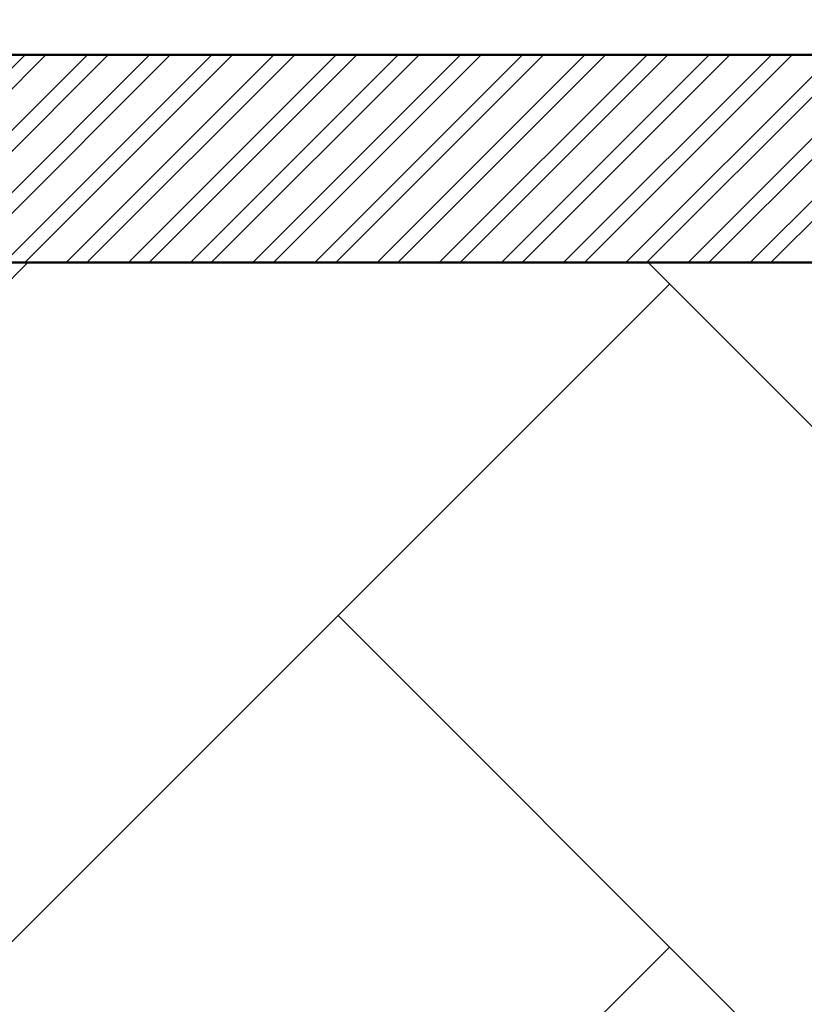
# Model space of a CAD drawing. Units: inches. Extents: x 3590 to 5167, y 65 to 1917.
# Tile 71 of 100: x 5001 to 5035, y 1765 to 1808. Entities that reach past the tile are written whole.
import ezdxf

# ---------------------------------------------------------------- set-up
doc = ezdxf.new("R2010")
doc.units = ezdxf.units.IN
for name, color, linetype, lineweight in [('A-ANNO-DIMS', 2, 'Continuous', 18), ('A-FLOR-PATT', 8, 'Continuous', 13), ('A-WALL', 7, 'Continuous', 50), ('A-WALL-PATT', 251, 'Continuous', 13)]:
    doc.layers.add(name, color=color, linetype=linetype, lineweight=lineweight)
doc.styles.get("Standard").update_dxf_attribs({"font": 'arial.ttf'})
doc.dimstyles.new('ISO-25', dxfattribs={"dimtxt": 9, "dimasz": 2.5, "dimexe": 1.25, "dimexo": 0.625, "dimtad": 1, "dimdec": 1, "dimlunit": 3, "dimtxsty": 'Standard', "dimcen": 2.5, "dimadec": 0, "dimazin": 0, "dimtfac": 1, "dimtdec": 1, "dimtmove": 0, "dimatfit": 3, "dimfxl": 1, "dimarcsym": 0})

# ---------------------------------------------------------------- blocks, each defined once
blk = doc.blocks.new('*D101')
at = {"layer": 'A-ANNO-DIMS', "color": 0, "lineweight": -2, "transparency": 16777216}
for p, q in [((4420.274, 1806.624), (4420.274, 1818.615)), ((5080.274, 1806.624), (5080.274, 1818.615)), ((4422.774, 1817.365), (5077.774, 1817.365))]:
    blk.add_line(p, q, dxfattribs=at)
at = {"layer": 'A-ANNO-DIMS', "color": 0, "transparency": 16777216}
for points in [[(4422.774, 1817.781), (4422.774, 1816.948), (4420.274, 1817.365)], [(5077.774, 1817.781), (5077.774, 1816.948), (5080.274, 1817.365)]]:
    blk.add_solid(points, dxfattribs=at)
at = {"layer": 'Defpoints', "color": 0, "transparency": 16777216}
for p in [(5080.274, 1817.365), (4420.274, 1805.999), (5080.274, 1805.999)]:
    blk.add_point(p, dxfattribs=at)
at = {"layer": 'A-ANNO-DIMS', "color": 0, "transparency": 16777216, "insert": (4750.274, 1822.566), "char_height": 9, "attachment_point": 5}
blk.add_mtext("55'", dxfattribs=at)

msp = doc.modelspace()

# ---------------------------------------------------------------- hatches: boundary and pattern name
at = {"layer": 'A-FLOR-PATT', "transparency": 33554687}
h = msp.add_hatch(dxfattribs=at)
h.set_pattern_fill('AR-HBONE', color=256, scale=0.2)
h.set_pattern_definition([(45, (-588.972, 0), (0, 28.73682), [60.96, -20.32]), (135, (-574.604, 14.368), (3e-15, 28.73682), [60.96, -20.32])])
h.paths.add_polyline_path([(5071.274, 1796.999), (4933.274, 1796.999), (4933.274, 1753.999), (4962.774, 1753.999, -0.414214), (4928.774, 1719.999), (4933.274, 1718.999), (4933.274, 1334.999), (5071.274, 1334.999)])
h.paths.add_polyline_path([(4951.78, 1521.077), (4951.715, 1521.04), (4951.563, 1520.895)], flags=16)
h.paths.add_polyline_path([(4952.267, 1521.376), (4952.198, 1521.371), (4952.198, 1521.356)], flags=0)
h.paths.add_polyline_path([(4967.051, 1529.728), (4965.231, 1528.694), (4963.411, 1527.714), (4961.756, 1526.851), (4963.589, 1527.449), (4964.036, 1527.478), (4962.975, 1527.249), (4961.76, 1526.852), (4959.792, 1525.834), (4958.005, 1524.895), (4956.24, 1523.93), (4954.504, 1522.919), (4954.129, 1522.682), (4953.361, 1521.997), (4953.366, 1521.998), (4953.605, 1522.064), (4955.106, 1522.761), (4956.921, 1523.434), (4958.678, 1523.915), (4960.358, 1524.2), (4961.945, 1524.286), (4964.171, 1524.108), (4965.958, 1523.309), (4963.863, 1522.976), (4965.187, 1522.499), (4963.366, 1522.497), (4961.545, 1522.487), (4959.764, 1522.461), (4958.304, 1522.419), (4957.974, 1522.388), (4956.307, 1522.232), (4954.718, 1522.071), (4953.251, 1521.899), (4953.525, 1521.623), (4954.331, 1521.379), (4956.243, 1521.23), (4958.039, 1520.93), (4959.684, 1520.483), (4961.16, 1519.896), (4963.107, 1518.8), (4964.393, 1517.325), (4962.973, 1517.726), (4964.558, 1516.661), (4965.407, 1515.708), (4963.507, 1516.322), (4961.68, 1517.005), (4959.935, 1517.745), (4958.282, 1518.528), (4956.732, 1519.343), (4955.295, 1520.175), (4954.672, 1520.572), (4954.513, 1520.627), (4955.658, 1519.318), (4956.703, 1517.982), (4957.644, 1516.647), (4958.485, 1515.334), (4959.55, 1513.524), (4960.438, 1511.769), (4958.841, 1513.62), (4957.452, 1515.325), (4955.819, 1517.459), (4956.665, 1515.448), (4957.111, 1513.923), (4957.447, 1511.714), (4957.076, 1509.793), (4956.538, 1511.11), (4955.992, 1512.569), (4955.444, 1514.125), (4954.898, 1515.735), (4954.357, 1517.356), (4953.824, 1518.943), (4953.305, 1520.452), (4953.065, 1521.116), (4952.971, 1521.146), (4952.949, 1521.086), (4952.73, 1520.199), (4953.37, 1518.024), (4953.757, 1516.373), (4954.051, 1514.765), (4954.264, 1513.221), (4954.471, 1511.131), (4954.497, 1510.402), (4954.409, 1511.76), (4954.264, 1513.221), (4954.051, 1514.765), (4953.757, 1516.373), (4953.37, 1518.024), (4952.877, 1519.698), (4952.716, 1520.141), (4952.533, 1519.059), (4952.374, 1517.789), (4952.219, 1516.312), (4952.046, 1514.6), (4951.833, 1512.626), (4951.557, 1510.363), (4951.203, 1512.168), (4950.852, 1514.339), (4950.985, 1516.376), (4951.66, 1518.286), (4952.593, 1520.481), (4952.357, 1521.13), (4951.855, 1520.328), (4950.839, 1518.908), (4949.777, 1517.587), (4948.916, 1516.617), (4948.111, 1515.256), (4947.089, 1513.554), (4945.889, 1511.615), (4946.326, 1513.402), (4946.562, 1514.249), (4945.528, 1513.327), (4944.581, 1512.531), (4946.018, 1514.508), (4947.204, 1516.048), (4947.893, 1517.313), (4949.307, 1518.764), (4950.414, 1519.767), (4950.451, 1519.806), (4952.267, 1521.376), (4951.645, 1521.493), (4950.404, 1521.18), (4948.044, 1520.359), (4946.119, 1519.452), (4944.572, 1518.475), (4943.35, 1517.443), (4941.997, 1515.92), (4941.661, 1515.275), (4942.813, 1516.99), (4944.572, 1518.475), (4946.119, 1519.452), (4948.044, 1520.359), (4950.404, 1521.18), (4951.645, 1521.493), (4949.647, 1521.868), (4948.6, 1521.756), (4947.126, 1521.57), (4945.42, 1521.348), (4943.45, 1521.105), (4941.183, 1520.856), (4942.86, 1521.613), (4943.873, 1522.03), (4942.952, 1521.909), (4941.41, 1521.485), (4939.543, 1520.67), (4938.968, 1520.226), (4940.733, 1521.299), (4942.952, 1521.909), (4943.702, 1522.008), (4945.894, 1522.7), (4947.565, 1522.714), (4948.921, 1522.566), (4951.131, 1522.183), (4950.971, 1522.297), (4948.129, 1523.006), (4946.035, 1523.707), (4944.232, 1524.521), (4942.707, 1525.461), (4941.444, 1526.537), (4940.43, 1527.761), (4939.649, 1529.143), (4941.421, 1528.122), (4943.147, 1527.132), (4944.841, 1526.175), (4946.514, 1525.25), (4948.179, 1524.359), (4948.365, 1524.263), (4946.475, 1526.045), (4945.181, 1527.54), (4944.19, 1529.033), (4943.496, 1530.54), (4943.278, 1531.36), (4942.498, 1531.919), (4943.114, 1531.762), (4942.959, 1533.659), (4944.14, 1531.989), (4944.612, 1531.323), (4946.202, 1530.463), (4947.486, 1529.509), (4948.79, 1528.226), (4950.368, 1526.237), (4949.485, 1528.155), (4948.851, 1530.123), (4948.491, 1532.041), (4948.381, 1533.918), (4948.501, 1535.76), (4948.827, 1537.573), (4949.418, 1535.565), (4949.957, 1533.569), (4950.464, 1531.586), (4950.961, 1529.617), (4951.391, 1527.954), (4951.724, 1530.687), (4952.201, 1532.58), (4952.889, 1534.33), (4953.77, 1535.951), (4954.827, 1537.46), (4954.521, 1535.39), (4954.273, 1533.937), (4955.58, 1535.663), (4956.748, 1536.739), (4956.159, 1534.78), (4955.589, 1532.873), (4955.043, 1531.006), (4954.525, 1529.166), (4954.038, 1527.341), (4953.638, 1525.733), (4953.611, 1525.586), (4953.398, 1524.166), (4953.382, 1524.009), (4954.07, 1525.476), (4954.912, 1527.022), (4956.136, 1528.894), (4957.847, 1530.577), (4959.376, 1531.54), (4958.256, 1530.104), (4957.143, 1528.663), (4956.066, 1527.243), (4955.056, 1525.871), (4954.141, 1524.571), (4953.352, 1523.372), (4953.311, 1523.303), (4953.273, 1522.925), (4953.261, 1522.382), (4954.103, 1523.373), (4954.63, 1524.284), (4955.961, 1526.358), (4957.23, 1528.13), (4958.421, 1529.609), (4960.037, 1531.368), (4961.374, 1532.375), (4962.101, 1532.77), (4961.07, 1531.061), (4959.987, 1529.438), (4958.869, 1527.908), (4958.15, 1527.007), (4959.803, 1528.003), (4961.589, 1528.793), (4963.391, 1529.328), (4965.211, 1529.632)], flags=16)
h.paths.add_polyline_path([(4962.944, 1523.182), (4961.107, 1523.422), (4960.392, 1523.362), (4962.35, 1523.331)], flags=0)
h.paths.add_polyline_path([(5049.541, 1584.551), (5049.476, 1584.515), (5049.325, 1584.37)], flags=16)
h.paths.add_polyline_path([(5050.028, 1584.851), (5049.959, 1584.845), (5049.959, 1584.83)], flags=0)
h.paths.add_polyline_path([(5042.333, 1581.949), (5043.88, 1582.926), (5045.806, 1583.833), (5048.165, 1584.654), (5049.406, 1584.967), (5047.408, 1585.342), (5046.361, 1585.231), (5044.888, 1585.044), (5043.181, 1584.822), (5041.211, 1584.579), (5038.944, 1584.33), (5040.622, 1585.087), (5041.634, 1585.504), (5040.713, 1585.383), (5039.171, 1584.959), (5037.304, 1584.144), (5036.729, 1583.7), (5038.494, 1584.773), (5040.713, 1585.383), (5041.463, 1585.482), (5043.655, 1586.174), (5045.326, 1586.188), (5046.682, 1586.04), (5048.893, 1585.657), (5048.732, 1585.771), (5045.891, 1586.48), (5043.796, 1587.181), (5041.994, 1587.996), (5040.468, 1588.935), (5039.205, 1590.011), (5038.191, 1591.235), (5037.41, 1592.617), (5039.182, 1591.596), (5040.909, 1590.607), (5042.602, 1589.649), (5044.275, 1588.724), (5045.94, 1587.833), (5046.126, 1587.738), (5044.237, 1589.519), (5042.942, 1591.015), (5041.952, 1592.508), (5041.257, 1594.014), (5041.039, 1594.834), (5040.26, 1595.393), (5040.875, 1595.237), (5040.721, 1597.133), (5041.901, 1595.463), (5042.373, 1594.798), (5043.963, 1593.938), (5045.247, 1592.983), (5046.552, 1591.701), (5048.129, 1589.712), (5047.247, 1591.63), (5046.613, 1593.597), (5046.252, 1595.515), (5046.142, 1597.392), (5046.262, 1599.234), (5046.588, 1601.047), (5047.179, 1599.039), (5047.718, 1597.043), (5048.225, 1595.06), (5048.722, 1593.091), (5049.152, 1591.429), (5049.485, 1594.161), (5049.962, 1596.054), (5050.65, 1597.804), (5051.532, 1599.425), (5052.589, 1600.934), (5052.283, 1598.864), (5052.034, 1597.411), (5053.341, 1599.137), (5054.509, 1600.213), (5053.92, 1598.254), (5053.35, 1596.348), (5052.805, 1594.48), (5052.286, 1592.64), (5051.799, 1590.815), (5051.4, 1589.207), (5051.373, 1589.06), (5051.159, 1587.64), (5051.143, 1587.483), (5051.831, 1588.95), (5052.673, 1590.496), (5053.898, 1592.368), (5055.608, 1594.051), (5057.137, 1595.014), (5056.017, 1593.578), (5054.904, 1592.137), (5053.828, 1590.717), (5052.817, 1589.345), (5051.902, 1588.046), (5051.113, 1586.846), (5051.072, 1586.777), (5051.034, 1586.399), (5051.022, 1585.856), (5051.864, 1586.847), (5052.391, 1587.758), (5053.723, 1589.832), (5054.991, 1591.604), (5056.182, 1593.083), (5057.798, 1594.842), (5059.135, 1595.849), (5059.863, 1596.244), (5058.831, 1594.535), (5057.749, 1592.912), (5056.63, 1591.382), (5055.912, 1590.482), (5057.564, 1591.477), (5059.35, 1592.267), (5061.152, 1592.802), (5062.972, 1593.106), (5064.812, 1593.203), (5062.992, 1592.169), (5061.172, 1591.188), (5059.518, 1590.325), (5061.35, 1590.924), (5061.797, 1590.952), (5060.737, 1590.723), (5059.521, 1590.326), (5057.553, 1589.308), (5055.766, 1588.369), (5054.002, 1587.404), (5052.265, 1586.393), (5051.891, 1586.156), (5051.122, 1585.471), (5051.127, 1585.472), (5051.366, 1585.538), (5052.867, 1586.235), (5054.682, 1586.908), (5056.439, 1587.389), (5058.12, 1587.675), (5059.706, 1587.76), (5061.933, 1587.583), (5063.719, 1586.783), (5061.624, 1586.45), (5062.949, 1585.973), (5061.127, 1585.971), (5059.307, 1585.961), (5057.525, 1585.935), (5056.065, 1585.893), (5055.735, 1585.862), (5054.068, 1585.707), (5052.479, 1585.546), (5051.012, 1585.373), (5051.286, 1585.097), (5052.092, 1584.853), (5054.004, 1584.704), (5055.8, 1584.404), (5057.446, 1583.958), (5058.921, 1583.37), (5060.868, 1582.274), (5062.154, 1580.799), (5060.734, 1581.2), (5062.32, 1580.135), (5063.168, 1579.182), (5061.269, 1579.796), (5059.441, 1580.479), (5057.696, 1581.219), (5056.043, 1582.003), (5054.493, 1582.817), (5053.057, 1583.649), (5052.433, 1584.047), (5052.274, 1584.101), (5053.42, 1582.793), (5054.464, 1581.457), (5055.405, 1580.121), (5056.247, 1578.809), (5057.311, 1576.998), (5058.199, 1575.244), (5056.602, 1577.094), (5055.213, 1578.799), (5053.58, 1580.933), (5054.427, 1578.922), (5054.872, 1577.397), (5055.208, 1575.189), (5054.838, 1573.267), (5054.299, 1574.584), (5053.754, 1576.043), (5053.206, 1577.599), (5052.659, 1579.209), (5052.118, 1580.83), (5051.585, 1582.417), (5051.066, 1583.927), (5050.826, 1584.59), (5050.733, 1584.62), (5050.711, 1584.561), (5050.491, 1583.673), (5051.131, 1581.498), (5051.518, 1579.847), (5051.813, 1578.24), (5052.026, 1576.695), (5052.233, 1574.605), (5052.258, 1573.876), (5052.17, 1575.234), (5052.026, 1576.695), (5051.813, 1578.24), (5051.518, 1579.847), (5051.131, 1581.498), (5050.638, 1583.172), (5050.477, 1583.615), (5050.294, 1582.533), (5050.136, 1581.263), (5049.981, 1579.786), (5049.807, 1578.074), (5049.594, 1576.1), (5049.318, 1573.837), (5048.965, 1575.642), (5048.613, 1577.813), (5048.747, 1579.85), (5049.421, 1581.76), (5050.354, 1583.955), (5050.118, 1584.604), (5049.616, 1583.802), (5048.6, 1582.382), (5047.538, 1581.061), (5046.677, 1580.091), (5045.872, 1578.73), (5044.85, 1577.028), (5043.651, 1575.089), (5044.087, 1576.877), (5044.324, 1577.723), (5043.289, 1576.801), (5042.342, 1576.005), (5043.779, 1577.982), (5044.966, 1579.522), (5045.655, 1580.787), (5047.068, 1582.239), (5048.175, 1583.241), (5048.213, 1583.28), (5050.028, 1584.851), (5049.406, 1584.967), (5048.165, 1584.654), (5045.806, 1583.833), (5043.88, 1582.926), (5042.333, 1581.949), (5041.111, 1580.917), (5039.758, 1579.394), (5039.423, 1578.749), (5040.575, 1580.464)], flags=16)
h.paths.add_polyline_path([(4954.799, 1533.12), (4954.262, 1532.079), (4953.831, 1530.935), (4953.505, 1529.636), (4953.283, 1528.133), (4953.167, 1526.376), (4953.156, 1524.315), (4953.277, 1521.236), (4952.802, 1521.842), (4951.557, 1521.998), (4950.976, 1521.961), (4952.661, 1521.941), (4952.802, 1521.842), (4953.152, 1523.593), (4953.167, 1526.376), (4953.283, 1528.133), (4953.609, 1530.346), (4954.456, 1532.592)], flags=0)
h.paths.add_polyline_path([(5050.563, 1585.316), (5049.318, 1585.472), (5048.737, 1585.435), (5050.422, 1585.415), (5050.563, 1585.316), (5050.914, 1587.067), (5050.928, 1589.851), (5051.045, 1591.607), (5051.371, 1593.82), (5052.217, 1596.066), (5052.56, 1596.594), (5052.024, 1595.554), (5051.592, 1594.409), (5051.266, 1593.11), (5051.045, 1591.607), (5050.928, 1589.851), (5050.918, 1587.789), (5051.038, 1584.71)], flags=0)
h.paths.add_polyline_path([(5058.153, 1586.836), (5060.111, 1586.805), (5060.705, 1586.656), (5058.868, 1586.896)], flags=0)
h.paths.add_polyline_path([(5049.541, 1430.936), (5049.476, 1430.9), (5049.325, 1430.755)], flags=16)
h.paths.add_polyline_path([(5050.028, 1431.236), (5049.959, 1431.231), (5049.959, 1431.215)], flags=0)
h.paths.add_polyline_path([(5046.588, 1447.432), (5047.179, 1445.425), (5047.718, 1443.429), (5048.225, 1441.446), (5048.722, 1439.476), (5049.152, 1437.814), (5049.485, 1440.546), (5049.962, 1442.439), (5050.65, 1444.189), (5051.532, 1445.811), (5052.589, 1447.319), (5052.283, 1445.249), (5052.034, 1443.796), (5053.341, 1445.522), (5054.509, 1446.598), (5053.92, 1444.64), (5053.35, 1442.733), (5052.805, 1440.865), (5052.286, 1439.025), (5051.799, 1437.201), (5051.4, 1435.592), (5051.373, 1435.445), (5051.159, 1434.025), (5051.143, 1433.868), (5051.831, 1435.335), (5052.673, 1436.881), (5053.898, 1438.753), (5055.608, 1440.436), (5057.137, 1441.4), (5056.017, 1439.963), (5054.904, 1438.522), (5053.828, 1437.102), (5052.817, 1435.73), (5051.902, 1434.431), (5051.113, 1433.231), (5051.072, 1433.162), (5051.034, 1432.784), (5051.022, 1432.242), (5051.864, 1433.232), (5052.391, 1434.143), (5053.723, 1436.217), (5054.991, 1437.989), (5056.182, 1439.468), (5057.798, 1441.227), (5059.135, 1442.235), (5059.863, 1442.629), (5058.831, 1440.921), (5057.749, 1439.298), (5056.63, 1437.767), (5055.912, 1436.867), (5057.564, 1437.863), (5059.35, 1438.652), (5061.152, 1439.187), (5062.972, 1439.491), (5064.812, 1439.588), (5062.992, 1438.554), (5061.172, 1437.573), (5059.518, 1436.71), (5061.35, 1437.309), (5061.797, 1437.337), (5060.737, 1437.108), (5059.521, 1436.711), (5057.553, 1435.693), (5055.766, 1434.754), (5054.002, 1433.789), (5052.265, 1432.778), (5051.891, 1432.541), (5051.122, 1431.856), (5051.127, 1431.857), (5051.366, 1431.923), (5052.867, 1432.62), (5054.682, 1433.293), (5056.439, 1433.775), (5058.12, 1434.06), (5059.706, 1434.145), (5061.933, 1433.968), (5063.719, 1433.168), (5061.624, 1432.835), (5062.949, 1432.358), (5061.127, 1432.357), (5059.307, 1432.346), (5057.525, 1432.32), (5056.065, 1432.278), (5055.735, 1432.248), (5054.068, 1432.092), (5052.479, 1431.931), (5051.012, 1431.759), (5051.286, 1431.482), (5052.092, 1431.238), (5054.004, 1431.089), (5055.8, 1430.789), (5057.446, 1430.343), (5058.921, 1429.755), (5060.868, 1428.66), (5062.154, 1427.185), (5060.734, 1427.585), (5062.32, 1426.52), (5063.168, 1425.567), (5061.269, 1426.181), (5059.441, 1426.865), (5057.696, 1427.604), (5056.043, 1428.388), (5054.493, 1429.202), (5053.057, 1430.034), (5052.433, 1430.432), (5052.274, 1430.487), (5053.42, 1429.178), (5054.464, 1427.842), (5055.405, 1426.506), (5056.247, 1425.194), (5057.311, 1423.383), (5058.199, 1421.629), (5056.602, 1423.479), (5055.213, 1425.184), (5053.58, 1427.318), (5054.427, 1425.307), (5054.872, 1423.782), (5055.208, 1421.574), (5054.838, 1419.652), (5054.299, 1420.97), (5053.754, 1422.428), (5053.206, 1423.984), (5052.659, 1425.595), (5052.118, 1427.215), (5051.585, 1428.802), (5051.066, 1430.312), (5050.826, 1430.975), (5050.733, 1431.005), (5050.711, 1430.946), (5050.491, 1430.058), (5051.131, 1427.883), (5051.518, 1426.232), (5051.813, 1424.625), (5052.026, 1423.081), (5052.233, 1420.991), (5052.258, 1420.261), (5052.17, 1421.619), (5052.026, 1423.081), (5051.813, 1424.625), (5051.518, 1426.232), (5051.131, 1427.883), (5050.638, 1429.558), (5050.477, 1430.001), (5050.294, 1428.918), (5050.136, 1427.648), (5049.981, 1426.171), (5049.807, 1424.459), (5049.594, 1422.485), (5049.318, 1420.222), (5048.965, 1422.028), (5048.613, 1424.199), (5048.747, 1426.235), (5049.421, 1428.146), (5050.354, 1430.34), (5050.118, 1430.989), (5049.616, 1430.187), (5048.6, 1428.768), (5047.538, 1427.446), (5046.677, 1426.477), (5045.872, 1425.116), (5044.85, 1423.413), (5043.651, 1421.474), (5044.087, 1423.262), (5044.324, 1424.109), (5043.289, 1423.186), (5042.342, 1422.391), (5043.779, 1424.368), (5044.966, 1425.907), (5045.655, 1427.173), (5047.068, 1428.624), (5048.175, 1429.627), (5048.213, 1429.666), (5050.028, 1431.236), (5049.406, 1431.353), (5048.165, 1431.039), (5045.806, 1430.218), (5043.88, 1429.311), (5042.333, 1428.334), (5041.111, 1427.302), (5039.758, 1425.779), (5039.423, 1425.134), (5040.575, 1426.849), (5042.333, 1428.334), (5043.88, 1429.311), (5045.806, 1430.218), (5048.165, 1431.039), (5049.406, 1431.353), (5047.408, 1431.727), (5046.361, 1431.616), (5044.888, 1431.429), (5043.181, 1431.207), (5041.211, 1430.964), (5038.944, 1430.715), (5040.622, 1431.472), (5041.634, 1431.89), (5040.713, 1431.769), (5039.171, 1431.345), (5037.304, 1430.53), (5036.729, 1430.085), (5038.494, 1431.158), (5040.713, 1431.769), (5041.463, 1431.867), (5043.655, 1432.559), (5045.326, 1432.573), (5046.682, 1432.425), (5048.893, 1432.042), (5048.732, 1432.156), (5045.891, 1432.865), (5043.796, 1433.566), (5041.994, 1434.381), (5040.468, 1435.321), (5039.205, 1436.396), (5038.191, 1437.62), (5037.41, 1439.002), (5039.182, 1437.982), (5040.909, 1436.992), (5042.602, 1436.034), (5044.275, 1435.109), (5045.94, 1434.218), (5046.126, 1434.123), (5044.237, 1435.904), (5042.942, 1437.4), (5041.952, 1438.893), (5041.257, 1440.399), (5041.039, 1441.219), (5040.26, 1441.778), (5040.875, 1441.622), (5040.721, 1443.518), (5041.901, 1441.848), (5042.373, 1441.183), (5043.963, 1440.323), (5045.247, 1439.369), (5046.552, 1438.086), (5048.129, 1436.097), (5047.247, 1438.015), (5046.613, 1439.982), (5046.252, 1441.901), (5046.142, 1443.778), (5046.262, 1445.619)], flags=16)
h.paths.add_polyline_path([(5052.382, 1444.255), (5051.623, 1442.78), (5052.024, 1441.939), (5052.56, 1442.98)], flags=0)
h.paths.add_polyline_path([(5050.563, 1431.701), (5049.318, 1431.857), (5048.737, 1431.821), (5050.422, 1431.8)], flags=0)
h.paths.add_polyline_path([(5058.153, 1433.221), (5060.111, 1433.19), (5060.705, 1433.041), (5058.868, 1433.281)], flags=0)
h.paths.add_polyline_path([(5049.541, 1352.285), (5049.476, 1352.249), (5049.325, 1352.104)], flags=16)
h.paths.add_polyline_path([(5050.028, 1352.585), (5049.959, 1352.58), (5049.959, 1352.564)], flags=0)
h.paths.add_polyline_path([(5046.588, 1368.781), (5047.179, 1366.774), (5047.718, 1364.778), (5048.225, 1362.795), (5048.722, 1360.825), (5049.152, 1359.163), (5049.485, 1361.896), (5049.962, 1363.789), (5050.65, 1365.538), (5051.532, 1367.16), (5052.589, 1368.669), (5052.283, 1366.598), (5052.034, 1365.145), (5053.341, 1366.871), (5054.509, 1367.947), (5053.92, 1365.989), (5053.35, 1364.082), (5052.805, 1362.214), (5052.286, 1360.374), (5051.799, 1358.55), (5051.4, 1356.942), (5051.373, 1356.794), (5051.159, 1355.374), (5051.143, 1355.218), (5051.831, 1356.684), (5052.673, 1358.23), (5053.898, 1360.102), (5055.608, 1361.786), (5057.137, 1362.749), (5056.017, 1361.313), (5054.904, 1359.872), (5053.828, 1358.452), (5052.817, 1357.079), (5051.902, 1355.78), (5051.113, 1354.581), (5051.072, 1354.512), (5051.034, 1354.133), (5051.022, 1353.591), (5051.864, 1354.581), (5052.391, 1355.492), (5053.723, 1357.566), (5054.991, 1359.338), (5056.182, 1360.817), (5057.798, 1362.577), (5059.135, 1363.584), (5059.863, 1363.979), (5058.831, 1362.27), (5057.749, 1360.647), (5056.63, 1359.117), (5055.912, 1358.216), (5057.564, 1359.212), (5059.35, 1360.001), (5061.152, 1360.536), (5062.972, 1360.841), (5064.812, 1360.937), (5062.992, 1359.903), (5061.172, 1358.923), (5059.518, 1358.059), (5061.35, 1358.658), (5061.797, 1358.687), (5060.737, 1358.458), (5059.521, 1358.061), (5057.553, 1357.043), (5055.766, 1356.103), (5054.002, 1355.138), (5052.265, 1354.127), (5051.891, 1353.89), (5051.122, 1353.206), (5051.127, 1353.206), (5051.366, 1353.272), (5052.867, 1353.969), (5054.682, 1354.643), (5056.439, 1355.124), (5058.12, 1355.409), (5059.706, 1355.495), (5061.933, 1355.317), (5063.719, 1354.518), (5061.624, 1354.184), (5062.949, 1353.708), (5061.127, 1353.706), (5059.307, 1353.695), (5057.525, 1353.669), (5056.065, 1353.627), (5055.735, 1353.597), (5054.068, 1353.441), (5052.479, 1353.28), (5051.012, 1353.108), (5051.286, 1352.831), (5052.092, 1352.587), (5054.004, 1352.439), (5055.8, 1352.138), (5057.446, 1351.692), (5058.921, 1351.104), (5060.868, 1350.009), (5062.154, 1348.534), (5060.734, 1348.935), (5062.32, 1347.869), (5063.168, 1346.916), (5061.269, 1347.53), (5059.441, 1348.214), (5057.696, 1348.954), (5056.043, 1349.737), (5054.493, 1350.551), (5053.057, 1351.383), (5052.433, 1351.781), (5052.274, 1351.836), (5053.42, 1350.527), (5054.464, 1349.191), (5055.405, 1347.855), (5056.247, 1346.543), (5057.311, 1344.733), (5058.199, 1342.978), (5056.602, 1344.828), (5055.213, 1346.534), (5053.58, 1348.667), (5054.427, 1346.656), (5054.872, 1345.132), (5055.208, 1342.923), (5054.838, 1341.002), (5054.299, 1342.319), (5053.754, 1343.778), (5053.206, 1345.334), (5052.659, 1346.944), (5052.118, 1348.564), (5051.585, 1350.151), (5051.066, 1351.661), (5050.826, 1352.324), (5050.733, 1352.355), (5050.711, 1352.295), (5050.491, 1351.408), (5051.131, 1349.232), (5051.518, 1347.581), (5051.813, 1345.974), (5052.026, 1344.43), (5052.233, 1342.34), (5052.258, 1341.61), (5052.17, 1342.969), (5052.026, 1344.43), (5051.813, 1345.974), (5051.518, 1347.581), (5051.131, 1349.232), (5050.638, 1350.907), (5050.477, 1351.35), (5050.294, 1350.267), (5050.136, 1348.997), (5049.981, 1347.52), (5049.807, 1345.809), (5049.594, 1343.835), (5049.318, 1341.571), (5048.965, 1343.377), (5048.613, 1345.548), (5048.747, 1347.585), (5049.421, 1349.495), (5050.354, 1351.689), (5050.118, 1352.339), (5049.616, 1351.536), (5048.6, 1350.117), (5047.538, 1348.795), (5046.677, 1347.826), (5045.872, 1346.465), (5044.85, 1344.763), (5043.651, 1342.824), (5044.087, 1344.611), (5044.324, 1345.458), (5043.289, 1344.535), (5042.342, 1343.74), (5043.779, 1345.717), (5044.966, 1347.256), (5045.655, 1348.522), (5047.068, 1349.973), (5048.175, 1350.976), (5048.213, 1351.015), (5050.028, 1352.585), (5049.406, 1352.702), (5048.165, 1352.388), (5045.806, 1351.567), (5043.88, 1350.661), (5042.333, 1349.683), (5041.111, 1348.651), (5039.758, 1347.128), (5039.423, 1346.483), (5040.575, 1348.198), (5042.333, 1349.683), (5043.88, 1350.661), (5045.806, 1351.567), (5048.165, 1352.388), (5049.406, 1352.702), (5047.408, 1353.076), (5046.361, 1352.965), (5044.888, 1352.779), (5043.181, 1352.556), (5041.211, 1352.313), (5038.944, 1352.065), (5040.622, 1352.821), (5041.634, 1353.239), (5040.713, 1353.118), (5039.171, 1352.694), (5037.304, 1351.879), (5036.729, 1351.434), (5038.494, 1352.508), (5040.713, 1353.118), (5041.463, 1353.216), (5043.655, 1353.909), (5045.326, 1353.923), (5046.682, 1353.774), (5048.893, 1353.391), (5048.732, 1353.506), (5045.891, 1354.214), (5043.796, 1354.915), (5041.994, 1355.73), (5040.468, 1356.67), (5039.205, 1357.746), (5038.191, 1358.969), (5037.41, 1360.352), (5039.182, 1359.331), (5040.909, 1358.341), (5042.602, 1357.383), (5044.275, 1356.458), (5045.94, 1355.567), (5046.126, 1355.472), (5044.237, 1357.253), (5042.942, 1358.749), (5041.952, 1360.242), (5041.257, 1361.748), (5041.039, 1362.568), (5040.26, 1363.128), (5040.875, 1362.971), (5040.721, 1364.867), (5041.901, 1363.197), (5042.373, 1362.532), (5043.963, 1361.672), (5045.247, 1360.718), (5046.552, 1359.435), (5048.129, 1357.446), (5047.247, 1359.364), (5046.613, 1361.331), (5046.252, 1363.25), (5046.142, 1365.127), (5046.262, 1366.969)], flags=16)
h.paths.add_polyline_path([(5052.382, 1365.604), (5051.623, 1364.129), (5052.024, 1363.288), (5052.56, 1364.329)], flags=0)
h.paths.add_polyline_path([(4951.78, 1698.041), (4951.715, 1698.005), (4951.563, 1697.859)], flags=16)
h.paths.add_polyline_path([(4952.267, 1698.341), (4952.198, 1698.335), (4952.198, 1698.32)], flags=0)
h.paths.add_polyline_path([(4957.076, 1686.757), (4956.538, 1688.074), (4955.992, 1689.533), (4955.444, 1691.089), (4954.898, 1692.699), (4954.357, 1694.32), (4953.824, 1695.907), (4953.305, 1697.417), (4953.065, 1698.08), (4952.971, 1698.11), (4952.949, 1698.051), (4952.73, 1697.163), (4953.37, 1694.988), (4953.757, 1693.337), (4954.051, 1691.729), (4954.264, 1690.185), (4954.471, 1688.095), (4954.497, 1687.366), (4954.409, 1688.724), (4954.264, 1690.185), (4954.051, 1691.729), (4953.757, 1693.337), (4953.37, 1694.988), (4952.877, 1696.662), (4952.716, 1697.105), (4952.533, 1696.023), (4952.374, 1694.753), (4952.219, 1693.276), (4952.046, 1691.564), (4951.833, 1689.59), (4951.557, 1687.327), (4951.203, 1689.132), (4950.852, 1691.303), (4950.985, 1693.34), (4951.66, 1695.25), (4952.593, 1697.445), (4952.357, 1698.094), (4951.855, 1697.292), (4950.839, 1695.872), (4949.777, 1694.551), (4948.916, 1693.581), (4948.111, 1692.22), (4947.089, 1690.518), (4945.889, 1688.579), (4946.326, 1690.366), (4946.562, 1691.213), (4945.528, 1690.291), (4944.581, 1689.495), (4946.018, 1691.472), (4947.204, 1693.012), (4947.893, 1694.277), (4949.307, 1695.729), (4950.414, 1696.731), (4950.451, 1696.77), (4952.267, 1698.341), (4951.645, 1698.457), (4950.404, 1698.144), (4948.044, 1697.323), (4946.119, 1696.416), (4944.572, 1695.439), (4943.35, 1694.407), (4941.997, 1692.884), (4941.661, 1692.239), (4942.813, 1693.954), (4944.572, 1695.439), (4946.119, 1696.416), (4948.044, 1697.323), (4950.404, 1698.144), (4951.645, 1698.457), (4949.647, 1698.832), (4948.6, 1698.72), (4947.126, 1698.534), (4945.42, 1698.312), (4943.45, 1698.069), (4941.183, 1697.82), (4942.86, 1698.577), (4943.873, 1698.994), (4942.952, 1698.873), (4941.41, 1698.449), (4939.543, 1697.634), (4938.968, 1697.19), (4940.733, 1698.263), (4942.952, 1698.873), (4943.702, 1698.972), (4945.894, 1699.664), (4947.565, 1699.678), (4948.921, 1699.53), (4951.131, 1699.147), (4950.971, 1699.261), (4948.129, 1699.97), (4946.035, 1700.671), (4944.232, 1701.486), (4942.707, 1702.425), (4941.444, 1703.501), (4940.43, 1704.725), (4939.649, 1706.107), (4941.421, 1705.086), (4943.147, 1704.097), (4944.841, 1703.139), (4946.514, 1702.214), (4948.179, 1701.323), (4948.365, 1701.227), (4946.475, 1703.009), (4945.181, 1704.505), (4944.19, 1705.997), (4943.496, 1707.504), (4943.278, 1708.324), (4942.498, 1708.883), (4943.114, 1708.727), (4942.959, 1710.623), (4944.14, 1708.953), (4944.612, 1708.287), (4946.202, 1707.428), (4947.486, 1706.473), (4948.79, 1705.191), (4950.368, 1703.202), (4949.485, 1705.12), (4948.851, 1707.087), (4948.491, 1709.005), (4948.381, 1710.882), (4948.501, 1712.724), (4948.827, 1714.537), (4949.418, 1712.529), (4949.957, 1710.533), (4950.464, 1708.55), (4950.961, 1706.581), (4951.391, 1704.919), (4951.724, 1707.651), (4952.201, 1709.544), (4952.889, 1711.294), (4953.77, 1712.915), (4954.827, 1714.424), (4954.521, 1712.354), (4954.273, 1710.901), (4955.58, 1712.627), (4956.748, 1713.703), (4956.159, 1711.744), (4955.589, 1709.837), (4955.043, 1707.97), (4954.525, 1706.13), (4954.038, 1704.305), (4953.638, 1702.697), (4953.611, 1702.55), (4953.398, 1701.13), (4953.382, 1700.973), (4954.07, 1702.44), (4954.912, 1703.986), (4956.136, 1705.858), (4957.847, 1707.541), (4959.376, 1708.504), (4958.256, 1707.068), (4957.143, 1705.627), (4956.066, 1704.207), (4955.056, 1702.835), (4954.141, 1701.536), (4953.352, 1700.336), (4953.311, 1700.267), (4953.273, 1699.889), (4953.261, 1699.346), (4954.103, 1700.337), (4954.63, 1701.248), (4955.961, 1703.322), (4957.23, 1705.094), (4958.421, 1706.573), (4960.037, 1708.332), (4961.374, 1709.339), (4962.101, 1709.734), (4961.07, 1708.025), (4959.987, 1706.402), (4958.869, 1704.872), (4958.15, 1703.972), (4959.803, 1704.967), (4961.589, 1705.757), (4963.391, 1706.292), (4965.211, 1706.596), (4967.051, 1706.692), (4965.231, 1705.659), (4963.411, 1704.678), (4961.756, 1703.815), (4963.589, 1704.413), (4964.036, 1704.442), (4962.975, 1704.213), (4961.76, 1703.816), (4959.792, 1702.798), (4958.005, 1701.859), (4956.24, 1700.894), (4954.504, 1699.883), (4954.129, 1699.646), (4953.361, 1698.961), (4953.366, 1698.962), (4953.605, 1699.028), (4955.106, 1699.725), (4956.921, 1700.398), (4958.678, 1700.879), (4960.358, 1701.164), (4961.945, 1701.25), (4964.171, 1701.073), (4965.958, 1700.273), (4963.863, 1699.94), (4965.187, 1699.463), (4963.366, 1699.461), (4961.545, 1699.451), (4959.764, 1699.425), (4958.304, 1699.383), (4957.974, 1699.352), (4956.307, 1699.197), (4954.718, 1699.036), (4953.251, 1698.863), (4953.525, 1698.587), (4954.331, 1698.343), (4956.243, 1698.194), (4958.039, 1697.894), (4959.684, 1697.447), (4961.16, 1696.86), (4963.107, 1695.764), (4964.393, 1694.289), (4962.973, 1694.69), (4964.558, 1693.625), (4965.407, 1692.672), (4963.507, 1693.286), (4961.68, 1693.969), (4959.935, 1694.709), (4958.282, 1695.492), (4956.732, 1696.307), (4955.295, 1697.139), (4954.672, 1697.536), (4954.513, 1697.591), (4955.658, 1696.282), (4956.703, 1694.946), (4957.644, 1693.611), (4958.485, 1692.298), (4959.55, 1690.488), (4960.438, 1688.733), (4958.841, 1690.584), (4957.452, 1692.289), (4955.819, 1694.423), (4956.665, 1692.412), (4957.111, 1690.887), (4957.447, 1688.678)], flags=16)
h.paths.add_polyline_path([(5050.563, 1353.05), (5049.318, 1353.207), (5048.737, 1353.17), (5050.422, 1353.15)], flags=0)
h.paths.add_polyline_path([(4951.78, 1351.486), (4951.715, 1351.45), (4951.563, 1351.305)], flags=16)
h.paths.add_polyline_path([(4952.267, 1351.786), (4952.198, 1351.78), (4952.198, 1351.765)], flags=0)
h.paths.add_polyline_path([(4954.827, 1367.869), (4954.521, 1365.799), (4954.273, 1364.346), (4955.58, 1366.072), (4956.748, 1367.148), (4956.159, 1365.19), (4955.589, 1363.283), (4955.043, 1361.415), (4954.525, 1359.575), (4954.038, 1357.751), (4953.638, 1356.142), (4953.611, 1355.995), (4953.398, 1354.575), (4953.382, 1354.418), (4954.07, 1355.885), (4954.912, 1357.431), (4956.136, 1359.303), (4957.847, 1360.986), (4959.376, 1361.95), (4958.256, 1360.513), (4957.143, 1359.072), (4956.066, 1357.652), (4955.056, 1356.28), (4954.141, 1354.981), (4953.352, 1353.781), (4953.311, 1353.712), (4953.273, 1353.334), (4953.261, 1352.792), (4954.103, 1353.782), (4954.63, 1354.693), (4955.961, 1356.767), (4957.23, 1358.539), (4958.421, 1360.018), (4960.037, 1361.777), (4961.374, 1362.785), (4962.101, 1363.179), (4961.07, 1361.471), (4959.987, 1359.848), (4958.869, 1358.317), (4958.15, 1357.417), (4959.803, 1358.413), (4961.589, 1359.202), (4963.391, 1359.737), (4965.211, 1360.041), (4967.051, 1360.138), (4965.231, 1359.104), (4963.411, 1358.123), (4961.756, 1357.26), (4963.589, 1357.859), (4964.036, 1357.887), (4962.975, 1357.658), (4961.76, 1357.261), (4959.792, 1356.243), (4958.005, 1355.304), (4956.24, 1354.339), (4954.504, 1353.328), (4954.129, 1353.091), (4953.361, 1352.406), (4953.366, 1352.407), (4953.605, 1352.473), (4955.106, 1353.17), (4956.921, 1353.843), (4958.678, 1354.325), (4960.358, 1354.61), (4961.945, 1354.695), (4964.171, 1354.518), (4965.958, 1353.718), (4963.863, 1353.385), (4965.187, 1352.908), (4963.366, 1352.907), (4961.545, 1352.896), (4959.764, 1352.87), (4958.304, 1352.828), (4957.974, 1352.798), (4956.307, 1352.642), (4954.718, 1352.481), (4953.251, 1352.309), (4953.525, 1352.032), (4954.331, 1351.788), (4956.243, 1351.639), (4958.039, 1351.339), (4959.684, 1350.893), (4961.16, 1350.305), (4963.107, 1349.21), (4964.393, 1347.735), (4962.973, 1348.135), (4964.558, 1347.07), (4965.407, 1346.117), (4963.507, 1346.731), (4961.68, 1347.414), (4959.935, 1348.154), (4958.282, 1348.938), (4956.732, 1349.752), (4955.295, 1350.584), (4954.672, 1350.982), (4954.513, 1351.036), (4955.658, 1349.728), (4956.703, 1348.392), (4957.644, 1347.056), (4958.485, 1345.744), (4959.55, 1343.933), (4960.438, 1342.179), (4958.841, 1344.029), (4957.452, 1345.734), (4955.819, 1347.868), (4956.665, 1345.857), (4957.111, 1344.332), (4957.447, 1342.124), (4957.076, 1340.202), (4956.538, 1341.52), (4955.992, 1342.978), (4955.444, 1344.534), (4954.898, 1346.145), (4954.357, 1347.765), (4953.824, 1349.352), (4953.305, 1350.862), (4953.065, 1351.525), (4952.971, 1351.555), (4952.949, 1351.496), (4952.73, 1350.608), (4953.37, 1348.433), (4953.757, 1346.782), (4954.051, 1345.175), (4954.264, 1343.631), (4954.471, 1341.541), (4954.497, 1340.811), (4954.409, 1342.169), (4954.264, 1343.631), (4954.051, 1345.175), (4953.757, 1346.782), (4953.37, 1348.433), (4952.877, 1350.108), (4952.716, 1350.551), (4952.533, 1349.468), (4952.374, 1348.198), (4952.219, 1346.721), (4952.046, 1345.009), (4951.833, 1343.035), (4951.557, 1340.772), (4951.203, 1342.578), (4950.852, 1344.749), (4950.985, 1346.785), (4951.66, 1348.696), (4952.593, 1350.89), (4952.357, 1351.539), (4951.855, 1350.737), (4950.839, 1349.318), (4949.777, 1347.996), (4948.916, 1347.027), (4948.111, 1345.665), (4947.089, 1343.963), (4945.889, 1342.024), (4946.326, 1343.812), (4946.562, 1344.659), (4945.528, 1343.736), (4944.581, 1342.941), (4946.018, 1344.918), (4947.204, 1346.457), (4947.893, 1347.723), (4949.307, 1349.174), (4950.414, 1350.177), (4950.451, 1350.216), (4952.267, 1351.786), (4951.645, 1351.903), (4950.404, 1351.589), (4948.044, 1350.768), (4946.119, 1349.861), (4944.572, 1348.884), (4943.35, 1347.852), (4941.997, 1346.329), (4941.661, 1345.684), (4942.813, 1347.399), (4944.572, 1348.884), (4946.119, 1349.861), (4948.044, 1350.768), (4950.404, 1351.589), (4951.645, 1351.903), (4949.647, 1352.277), (4948.6, 1352.166), (4947.126, 1351.979), (4945.42, 1351.757), (4943.45, 1351.514), (4941.183, 1351.265), (4942.86, 1352.022), (4943.873, 1352.44), (4942.952, 1352.319), (4941.41, 1351.895), (4939.543, 1351.08), (4938.968, 1350.635), (4940.733, 1351.708), (4942.952, 1352.319), (4943.702, 1352.417), (4945.894, 1353.109), (4947.565, 1353.123), (4948.921, 1352.975), (4951.131, 1352.592), (4950.971, 1352.706), (4948.129, 1353.415), (4946.035, 1354.116), (4944.232, 1354.931), (4942.707, 1355.871), (4941.444, 1356.946), (4940.43, 1358.17), (4939.649, 1359.552), (4941.421, 1358.532), (4943.147, 1357.542), (4944.841, 1356.584), (4946.514, 1355.659), (4948.179, 1354.768), (4948.365, 1354.673), (4946.475, 1356.454), (4945.181, 1357.95), (4944.19, 1359.443), (4943.496, 1360.949), (4943.278, 1361.769), (4942.498, 1362.328), (4943.114, 1362.172), (4942.959, 1364.068), (4944.14, 1362.398), (4944.612, 1361.733), (4946.202, 1360.873), (4947.486, 1359.919), (4948.79, 1358.636), (4950.368, 1356.647), (4949.485, 1358.565), (4948.851, 1360.532), (4948.491, 1362.451), (4948.381, 1364.328), (4948.501, 1366.169), (4948.827, 1367.982), (4949.418, 1365.975), (4949.957, 1363.979), (4950.464, 1361.995), (4950.961, 1360.026), (4951.391, 1358.364), (4951.724, 1361.096), (4952.201, 1362.989), (4952.889, 1364.739), (4953.77, 1366.361)], flags=16)
h.paths.add_polyline_path([(4954.799, 1363.53), (4954.262, 1362.489), (4953.831, 1361.344), (4953.505, 1360.045), (4953.283, 1358.543), (4953.167, 1356.786), (4953.156, 1354.724), (4953.277, 1351.646), (4952.802, 1352.251), (4951.557, 1352.407), (4950.976, 1352.371), (4952.661, 1352.35), (4952.802, 1352.251), (4953.152, 1354.002), (4953.167, 1356.786), (4953.283, 1358.543), (4953.609, 1360.755), (4954.456, 1363.001)], flags=0)
h.paths.add_polyline_path([(4952.802, 1698.806), (4951.557, 1698.962), (4950.976, 1698.925), (4952.661, 1698.905), (4952.802, 1698.806), (4953.152, 1700.557), (4953.167, 1703.34), (4953.283, 1705.097), (4953.609, 1707.31), (4954.456, 1709.556), (4954.799, 1710.084), (4954.262, 1709.043), (4953.831, 1707.899), (4953.505, 1706.6), (4953.283, 1705.097), (4953.167, 1703.34), (4953.156, 1701.279), (4953.277, 1698.2)], flags=0)
h.paths.add_polyline_path([(4962.944, 1700.146), (4961.107, 1700.386), (4960.392, 1700.326), (4962.35, 1700.295)], flags=0)
h.paths.add_polyline_path([(5058.153, 1354.57), (5060.111, 1354.539), (5060.705, 1354.391), (5058.868, 1354.631)], flags=0)
h.paths.add_polyline_path([(4962.944, 1353.591), (4961.107, 1353.831), (4960.392, 1353.771), (4962.35, 1353.74)], flags=0)
h.paths.add_polyline_path([(5049.541, 1778.72), (5049.476, 1778.684), (5049.325, 1778.539)], flags=16)
h.paths.add_polyline_path([(5050.028, 1779.02), (5049.959, 1779.014), (5049.959, 1778.999)], flags=0)
h.paths.add_polyline_path([(5052.258, 1768.045), (5052.17, 1769.403), (5052.026, 1770.864), (5051.813, 1772.409), (5051.518, 1774.016), (5051.131, 1775.667), (5050.638, 1777.341), (5050.477, 1777.784), (5050.294, 1776.702), (5050.136, 1775.432), (5049.981, 1773.955), (5049.807, 1772.243), (5049.594, 1770.269), (5049.318, 1768.006), (5048.965, 1769.811), (5048.613, 1771.982), (5048.747, 1774.019), (5049.421, 1775.929), (5050.354, 1778.124), (5050.118, 1778.773), (5049.616, 1777.971), (5048.6, 1776.551), (5047.538, 1775.23), (5046.677, 1774.26), (5045.872, 1772.899), (5044.85, 1771.197), (5043.651, 1769.258), (5044.087, 1771.046), (5044.324, 1771.892), (5043.289, 1770.97), (5042.342, 1770.174), (5043.779, 1772.151), (5044.966, 1773.691), (5045.655, 1774.956), (5047.068, 1776.408), (5048.175, 1777.41), (5048.213, 1777.449), (5050.028, 1779.02), (5049.406, 1779.136), (5048.165, 1778.823), (5045.806, 1778.002), (5043.88, 1777.095), (5042.333, 1776.118), (5041.111, 1775.086), (5039.758, 1773.563), (5039.423, 1772.918), (5040.575, 1774.633), (5042.333, 1776.118), (5043.88, 1777.095), (5045.806, 1778.002), (5048.165, 1778.823), (5049.406, 1779.136), (5047.408, 1779.511), (5046.361, 1779.4), (5044.888, 1779.213), (5043.181, 1778.991), (5041.211, 1778.748), (5038.944, 1778.499), (5040.622, 1779.256), (5041.634, 1779.673), (5040.713, 1779.552), (5039.171, 1779.128), (5037.304, 1778.313), (5036.729, 1777.869), (5038.494, 1778.942), (5040.713, 1779.552), (5041.463, 1779.651), (5043.655, 1780.343), (5045.326, 1780.357), (5046.682, 1780.209), (5048.893, 1779.826), (5048.732, 1779.94), (5045.891, 1780.649), (5043.796, 1781.35), (5041.994, 1782.165), (5040.468, 1783.104), (5039.205, 1784.18), (5038.191, 1785.404), (5037.41, 1786.786), (5039.182, 1785.765), (5040.909, 1784.776), (5042.602, 1783.818), (5044.275, 1782.893), (5045.94, 1782.002), (5046.126, 1781.907), (5044.237, 1783.688), (5042.942, 1785.184), (5041.952, 1786.677), (5041.257, 1788.183), (5041.039, 1789.003), (5040.26, 1789.562), (5040.875, 1789.406), (5040.721, 1791.302), (5041.901, 1789.632), (5042.373, 1788.967), (5043.963, 1788.107), (5045.247, 1787.152), (5046.552, 1785.87), (5048.129, 1783.881), (5047.247, 1785.799), (5046.613, 1787.766), (5046.252, 1789.684), (5046.142, 1791.561), (5046.262, 1793.403), (5046.588, 1795.216), (5047.179, 1793.208), (5047.718, 1791.213), (5048.225, 1789.229), (5048.722, 1787.26), (5049.152, 1785.598), (5049.485, 1788.33), (5049.962, 1790.223), (5050.65, 1791.973), (5051.532, 1793.594), (5052.589, 1795.103), (5052.283, 1793.033), (5052.034, 1791.58), (5053.341, 1793.306), (5054.509, 1794.382), (5053.92, 1792.423), (5053.35, 1790.517), (5052.805, 1788.649), (5052.286, 1786.809), (5051.799, 1784.984), (5051.4, 1783.376), (5051.373, 1783.229), (5051.159, 1781.809), (5051.143, 1781.652), (5051.831, 1783.119), (5052.673, 1784.665), (5053.898, 1786.537), (5055.608, 1788.22), (5057.137, 1789.183), (5056.017, 1787.747), (5054.904, 1786.306), (5053.828, 1784.886), (5052.817, 1783.514), (5051.902, 1782.215), (5051.113, 1781.015), (5051.072, 1780.946), (5051.034, 1780.568), (5051.022, 1780.025), (5051.864, 1781.016), (5052.391, 1781.927), (5053.723, 1784.001), (5054.991, 1785.773), (5056.182, 1787.252), (5057.798, 1789.011), (5059.135, 1790.018), (5059.863, 1790.413), (5058.831, 1788.704), (5057.749, 1787.081), (5056.63, 1785.551), (5055.912, 1784.651), (5057.564, 1785.646), (5059.35, 1786.436), (5061.152, 1786.971), (5062.972, 1787.275), (5064.812, 1787.372), (5062.992, 1786.338), (5061.172, 1785.357), (5059.518, 1784.494), (5061.35, 1785.093), (5061.797, 1785.121), (5060.737, 1784.892), (5059.521, 1784.495), (5057.553, 1783.477), (5055.766, 1782.538), (5054.002, 1781.573), (5052.265, 1780.562), (5051.891, 1780.325), (5051.122, 1779.64), (5051.127, 1779.641), (5051.366, 1779.707), (5052.867, 1780.404), (5054.682, 1781.077), (5056.439, 1781.558), (5058.12, 1781.844), (5059.706, 1781.929), (5061.933, 1781.752), (5063.719, 1780.952), (5061.624, 1780.619), (5062.949, 1780.142), (5061.127, 1780.14), (5059.307, 1780.13), (5057.525, 1780.104), (5056.065, 1780.062), (5055.735, 1780.031), (5054.068, 1779.876), (5052.479, 1779.715), (5051.012, 1779.542), (5051.286, 1779.266), (5052.092, 1779.022), (5054.004, 1778.873), (5055.8, 1778.573), (5057.446, 1778.127), (5058.921, 1777.539), (5060.868, 1776.443), (5062.154, 1774.968), (5060.734, 1775.369), (5062.32, 1774.304), (5063.168, 1773.351), (5061.269, 1773.965), (5059.441, 1774.648), (5057.696, 1775.388), (5056.043, 1776.172), (5054.493, 1776.986), (5053.057, 1777.818), (5052.433, 1778.216), (5052.274, 1778.27), (5053.42, 1776.962), (5054.464, 1775.626), (5055.405, 1774.29), (5056.247, 1772.978), (5057.311, 1771.167), (5058.199, 1769.413), (5056.602, 1771.263), (5055.213, 1772.968), (5053.58, 1775.102), (5054.427, 1773.091), (5054.872, 1771.566), (5055.208, 1769.358), (5054.838, 1767.436), (5054.299, 1768.753), (5053.754, 1770.212), (5053.206, 1771.768), (5052.659, 1773.378), (5052.118, 1774.999), (5051.585, 1776.586), (5051.066, 1778.096), (5050.826, 1778.759), (5050.733, 1778.789), (5050.711, 1778.73), (5050.491, 1777.842), (5051.131, 1775.667), (5051.518, 1774.016), (5051.813, 1772.409), (5052.026, 1770.864), (5052.233, 1768.774)], flags=16)
h.paths.add_polyline_path([(5050.563, 1779.485), (5049.318, 1779.641), (5048.737, 1779.604), (5050.422, 1779.584), (5050.563, 1779.485), (5050.914, 1781.236), (5050.928, 1784.02), (5051.045, 1785.776), (5051.371, 1787.989), (5052.217, 1790.235), (5052.56, 1790.763), (5052.024, 1789.723), (5051.592, 1788.578), (5051.266, 1787.279), (5051.045, 1785.776), (5050.928, 1784.02), (5050.918, 1781.958), (5051.038, 1778.879)], flags=0)
h.paths.add_polyline_path([(5058.153, 1781.005), (5060.111, 1780.974), (5060.705, 1780.825), (5058.868, 1781.065)], flags=0)
at = {"layer": 'A-WALL-PATT', "transparency": 33554687}
h = msp.add_hatch(dxfattribs=at)
h.set_pattern_fill('ANSI32', color=256, scale=0.2)
h.paths.add_polyline_path([(4684.274, 1805.999), (4591.274, 1805.999), (4591.274, 1796.999), (4639.274, 1796.999), (4639.274, 1790.999), (4648.274, 1790.999), (4648.274, 1796.999), (4684.274, 1796.999)])
h.paths.add_polyline_path([(4543.274, 1805.999), (4420.274, 1805.999), (4420.274, 1784.999), (4429.274, 1784.999), (4429.274, 1796.999), (4445.919, 1796.999), (4543.274, 1796.999)])
h.paths.add_polyline_path([(4828.274, 1805.999), (4744.274, 1805.999), (4744.274, 1796.999), (4828.274, 1796.999)])
h.paths.add_polyline_path([(4648.274, 1754.999), (4639.274, 1754.999), (4639.274, 1655.999), (4546.274, 1655.999), (4546.274, 1649.999), (4549.274, 1649.999), (4549.274, 1553.999), (4429.274, 1553.999), (4429.274, 1583.999), (4420.274, 1583.999), (4420.274, 1538.999), (4429.274, 1538.999), (4429.274, 1544.999), (4639.274, 1544.999), (4639.274, 1538.999), (4648.274, 1538.999), (4648.274, 1559.999), (4639.274, 1559.999), (4639.274, 1553.999), (4555.274, 1553.999), (4555.274, 1649.999), (4639.274, 1649.999), (4639.274, 1589.999), (4648.274, 1589.999)])
h.paths.add_polyline_path([(4516.274, 1655.999), (4429.274, 1655.999), (4429.274, 1736.999), (4420.274, 1736.999), (4420.274, 1619.999), (4429.274, 1619.999), (4429.274, 1649.999), (4516.274, 1649.999)], flags=17)
h.paths.add_polyline_path([(5080.274, 1805.999), (4888.274, 1805.999), (4888.274, 1796.999), (4924.274, 1796.999), (4924.274, 1754.999), (4933.274, 1754.999), (4933.274, 1796.999), (5071.274, 1796.999), (5071.274, 1334.999), (4933.274, 1334.999), (4933.274, 1565.999), (4924.274, 1565.999), (4924.274, 1334.999), (4898.774, 1334.999), (4898.774, 1325.999), (5080.274, 1325.999)])
h.paths.add_polyline_path([(4933.274, 1718.999), (4924.274, 1718.999), (4924.274, 1637.999), (4933.274, 1637.999)], flags=17)
h.paths.add_polyline_path([(4802.774, 1334.999), (4777.274, 1334.999), (4777.274, 1502.999), (4756.274, 1502.999), (4756.274, 1493.999), (4768.274, 1493.999), (4768.274, 1430.999), (4696.274, 1430.999), (4696.274, 1493.999), (4708.274, 1493.999), (4708.274, 1502.999), (4639.274, 1502.999), (4639.274, 1493.999), (4687.274, 1493.999), (4687.274, 1430.999), (4681.274, 1430.999), (4681.274, 1421.999), (4768.274, 1421.999), (4768.274, 1334.999), (4726.274, 1334.999), (4726.274, 1325.999), (4802.774, 1325.999)])
h.paths.add_polyline_path([(4690.274, 1334.999), (4648.274, 1334.999), (4648.274, 1352.867), (4648.274, 1421.999), (4651.274, 1421.999), (4651.274, 1430.999), (4639.274, 1430.999), (4639.274, 1334.999), (4633.274, 1334.999), (4633.274, 1325.999), (4690.274, 1325.999)])
h.paths.add_polyline_path([(4585.274, 1334.999), (4584.724, 1334.999), (4429.274, 1334.999), (4429.274, 1490.999), (4420.274, 1490.999), (4420.274, 1325.999), (4585.274, 1325.999)])

# ---------------------------------------------------------------- linework, layer by layer
at = {"layer": 'A-WALL'}
msp.add_line((4933.274, 1796.999), (5071.274, 1796.999), dxfattribs=at)
msp.add_lwpolyline([(5080.274, 1805.999), (5080.274, 1325.999), (4420.274, 1325.999), (4420.274, 1805.999)], close=True, dxfattribs=at)

# ---------------------------------------------------------------- dimensions: what is measured, and where the dimension line sits
at = {"layer": 'A-ANNO-DIMS'}
dim = msp.add_linear_dim(base=(5080.274, 1817.365), p1=(4420.274, 1805.999), p2=(5080.274, 1805.999), dimstyle='ISO-25', override={"dimclrd": 0, "dimclre": 0, "dimclrt": 0}, dxfattribs=at)
dim.commit()
dim.dimension.update_dxf_attribs({"geometry": '*D101', "text_midpoint": (4750.274, 1822.566)})

doc.saveas('drawing.dxf')
